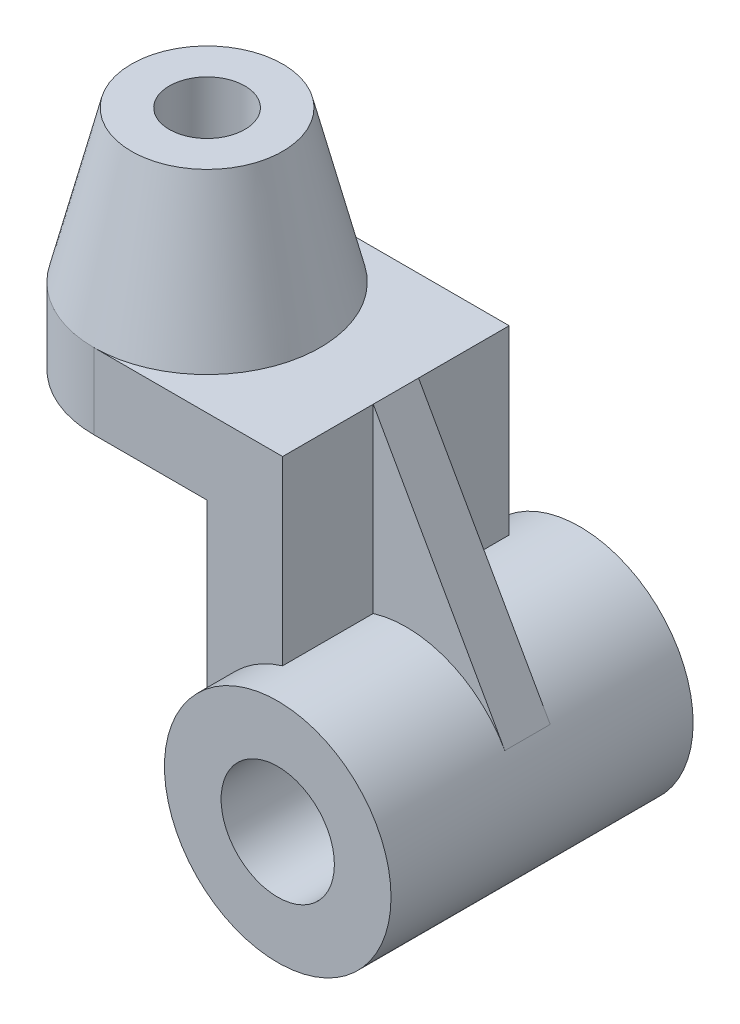
ISO-10303-21;
HEADER;
FILE_DESCRIPTION(('STEP AP214'),'2;1');
FILE_NAME('part.step','',(''),(''),'','','');
FILE_SCHEMA(('AUTOMOTIVE_DESIGN { 1 0 10303 214 1 1 1 1 }'));
ENDSEC;
DATA;
#1=APPLICATION_CONTEXT('core data for automotive mechanical design processes');
#2=APPLICATION_PROTOCOL_DEFINITION('international standard','automotive_design',2000,#1);
#3=PRODUCT_CONTEXT('',#1,'mechanical');
#4=PRODUCT('Part','Part','',(#3));
#5=PRODUCT_RELATED_PRODUCT_CATEGORY('part','',(#4));
#6=PRODUCT_DEFINITION_FORMATION('','',#4);
#7=PRODUCT_DEFINITION_CONTEXT('part definition',#1,'design');
#8=PRODUCT_DEFINITION('design','',#6,#7);
#9=PRODUCT_DEFINITION_SHAPE('','',#8);
#10=(LENGTH_UNIT() NAMED_UNIT(*) SI_UNIT(.MILLI.,.METRE.));
#11=(NAMED_UNIT(*) PLANE_ANGLE_UNIT() SI_UNIT($,.RADIAN.));
#12=(NAMED_UNIT(*) SI_UNIT($,.STERADIAN.) SOLID_ANGLE_UNIT());
#13=UNCERTAINTY_MEASURE_WITH_UNIT(LENGTH_MEASURE(1.E-05),#10,'distance_accuracy_value','');
#14=(GEOMETRIC_REPRESENTATION_CONTEXT(3) GLOBAL_UNCERTAINTY_ASSIGNED_CONTEXT((#13)) GLOBAL_UNIT_ASSIGNED_CONTEXT((#10,
#11,#12)) REPRESENTATION_CONTEXT('',''));
#15=CARTESIAN_POINT('',(0.,0.,0.));
#16=DIRECTION('',(0.,0.,1.));
#17=DIRECTION('',(1.,0.,0.));
#18=AXIS2_PLACEMENT_3D('',#15,#16,#17);
#19=CARTESIAN_POINT('',(-88.7082869338697,76.7082869338697,30.));
#20=DIRECTION('',(0.,-1.,0.));
#21=DIRECTION('',(1.,0.,0.));
#22=AXIS2_PLACEMENT_3D('',#19,#20,#21);
#23=PLANE('',#22);
#24=CARTESIAN_POINT('',(-58.7082869338697,76.7082869338697,0.));
#25=DIRECTION('',(0.,1.,0.));
#26=DIRECTION('',(-1.,0.,0.));
#27=AXIS2_PLACEMENT_3D('',#24,#25,#26);
#28=CIRCLE('',#27,30.);
#29=CARTESIAN_POINT('',(-58.7082869338697,76.7082869338697,30.));
#30=VERTEX_POINT('',#29);
#31=CARTESIAN_POINT('',(-58.7082869338697,76.7082869338697,-30.));
#32=VERTEX_POINT('',#31);
#33=EDGE_CURVE('E126',#30,#32,#28,.T.);
#34=ORIENTED_EDGE('',*,*,#33,.F.);
#35=DIRECTION('',(-1.,0.,0.));
#36=VECTOR('',#35,1.);
#37=CARTESIAN_POINT('',(-88.7082869338697,76.7082869338697,30.));
#38=LINE('',#37,#36);
#39=CARTESIAN_POINT('',(-8.7082869338697,76.7082869338697,30.));
#40=VERTEX_POINT('',#39);
#41=EDGE_CURVE('E109',#40,#30,#38,.T.);
#42=ORIENTED_EDGE('',*,*,#41,.F.);
#43=DIRECTION('',(0.,0.,-1.));
#44=VECTOR('',#43,1.);
#45=CARTESIAN_POINT('',(-8.7082869338697,76.7082869338697,30.));
#46=LINE('',#45,#44);
#47=CARTESIAN_POINT('',(-8.7082869338697,76.7082869338697,6.));
#48=VERTEX_POINT('',#47);
#49=EDGE_CURVE('E183',#40,#48,#46,.T.);
#50=ORIENTED_EDGE('',*,*,#49,.T.);
#51=DIRECTION('',(0.,0.,-1.));
#52=VECTOR('',#51,1.);
#53=CARTESIAN_POINT('',(-8.7082869338697,76.7082869338697,6.));
#54=LINE('',#53,#52);
#55=CARTESIAN_POINT('',(-8.7082869338697,76.7082869338697,-6.));
#56=VERTEX_POINT('',#55);
#57=EDGE_CURVE('E147',#48,#56,#54,.T.);
#58=ORIENTED_EDGE('',*,*,#57,.T.);
#59=CARTESIAN_POINT('',(-8.7082869338697,76.7082869338697,-30.));
#60=VERTEX_POINT('',#59);
#61=EDGE_CURVE('E184',#56,#60,#46,.T.);
#62=ORIENTED_EDGE('',*,*,#61,.T.);
#63=DIRECTION('',(-1.,0.,0.));
#64=VECTOR('',#63,1.);
#65=CARTESIAN_POINT('',(-88.7082869338697,76.7082869338697,-30.));
#66=LINE('',#65,#64);
#67=EDGE_CURVE('E128',#60,#32,#66,.T.);
#68=ORIENTED_EDGE('',*,*,#67,.T.);
#69=EDGE_LOOP('',(#34,#42,#50,#58,#62,#68));
#70=FACE_BOUND('',#69,.T.);
#71=ADVANCED_FACE('F39',(#70),#23,.F.);
#72=CARTESIAN_POINT('',(-28.7082869338697,56.7082869338697,30.));
#73=DIRECTION('',(0.,1.,0.));
#74=DIRECTION('',(-1.,0.,0.));
#75=AXIS2_PLACEMENT_3D('',#72,#73,#74);
#76=PLANE('',#75);
#77=CARTESIAN_POINT('',(-58.7082869338697,56.7082869338697,0.));
#78=DIRECTION('',(0.,1.,0.));
#79=DIRECTION('',(-1.,0.,0.));
#80=AXIS2_PLACEMENT_3D('',#77,#78,#79);
#81=CIRCLE('',#80,10.);
#82=CARTESIAN_POINT('',(-68.7082869338697,56.7082869338697,0.));
#83=VERTEX_POINT('',#82);
#84=EDGE_CURVE('E133',#83,#83,#81,.T.);
#85=ORIENTED_EDGE('',*,*,#84,.T.);
#86=EDGE_LOOP('',(#85));
#87=FACE_BOUND('',#86,.T.);
#88=CARTESIAN_POINT('',(-58.7082869338697,56.7082869338697,0.));
#89=DIRECTION('',(0.,1.,0.));
#90=DIRECTION('',(-1.,0.,0.));
#91=AXIS2_PLACEMENT_3D('',#88,#89,#90);
#92=CIRCLE('',#91,30.);
#93=CARTESIAN_POINT('',(-58.7082869338697,56.7082869338697,-30.));
#94=VERTEX_POINT('',#93);
#95=CARTESIAN_POINT('',(-58.7082869338697,56.7082869338697,30.));
#96=VERTEX_POINT('',#95);
#97=EDGE_CURVE('E53',#94,#96,#92,.T.);
#98=ORIENTED_EDGE('',*,*,#97,.F.);
#99=DIRECTION('',(1.,0.,0.));
#100=VECTOR('',#99,1.);
#101=CARTESIAN_POINT('',(-28.7082869338697,56.7082869338697,-30.));
#102=LINE('',#101,#100);
#103=CARTESIAN_POINT('',(-28.7082869338697,56.7082869338697,-30.));
#104=VERTEX_POINT('',#103);
#105=EDGE_CURVE('E177',#94,#104,#102,.T.);
#106=ORIENTED_EDGE('',*,*,#105,.T.);
#107=DIRECTION('',(0.,0.,-1.));
#108=VECTOR('',#107,1.);
#109=CARTESIAN_POINT('',(-28.7082869338697,56.7082869338697,30.));
#110=LINE('',#109,#108);
#111=CARTESIAN_POINT('',(-28.7082869338697,56.7082869338697,30.));
#112=VERTEX_POINT('',#111);
#113=EDGE_CURVE('E182',#112,#104,#110,.T.);
#114=ORIENTED_EDGE('',*,*,#113,.F.);
#115=DIRECTION('',(1.,0.,0.));
#116=VECTOR('',#115,1.);
#117=CARTESIAN_POINT('',(-28.7082869338697,56.7082869338697,30.));
#118=LINE('',#117,#116);
#119=EDGE_CURVE('E116',#96,#112,#118,.T.);
#120=ORIENTED_EDGE('',*,*,#119,.F.);
#121=EDGE_LOOP('',(#98,#106,#114,#120));
#122=FACE_BOUND('',#121,.T.);
#123=ADVANCED_FACE('F230',(#87,#122),#76,.F.);
#124=CARTESIAN_POINT('',(-8.7082869338697,76.7082869338697,30.));
#125=DIRECTION('',(-1.,0.,0.));
#126=DIRECTION('',(0.,-1.,0.));
#127=AXIS2_PLACEMENT_3D('',#124,#125,#126);
#128=PLANE('',#127);
#129=DIRECTION('',(0.,-1.,0.));
#130=VECTOR('',#129,1.);
#131=CARTESIAN_POINT('',(-8.7082869338697,76.7082869338697,-6.));
#132=LINE('',#131,#130);
#133=CARTESIAN_POINT('',(-8.7082869338697,28.7082869338697,-6.));
#134=VERTEX_POINT('',#133);
#135=EDGE_CURVE('E140',#56,#134,#132,.T.);
#136=ORIENTED_EDGE('',*,*,#135,.T.);
#137=DIRECTION('',(0.,0.,-1.));
#138=VECTOR('',#137,1.);
#139=CARTESIAN_POINT('',(-8.7082869338697,28.7082869338697,30.));
#140=LINE('',#139,#138);
#141=CARTESIAN_POINT('',(-8.7082869338697,28.7082869338697,-30.));
#142=VERTEX_POINT('',#141);
#143=EDGE_CURVE('E190',#134,#142,#140,.T.);
#144=ORIENTED_EDGE('',*,*,#143,.T.);
#145=DIRECTION('',(0.,1.,0.));
#146=VECTOR('',#145,1.);
#147=CARTESIAN_POINT('',(-8.7082869338697,76.7082869338697,-30.));
#148=LINE('',#147,#146);
#149=EDGE_CURVE('E175',#142,#60,#148,.T.);
#150=ORIENTED_EDGE('',*,*,#149,.T.);
#151=ORIENTED_EDGE('',*,*,#61,.F.);
#152=EDGE_LOOP('',(#136,#144,#150,#151));
#153=FACE_BOUND('',#152,.T.);
#154=ADVANCED_FACE('F225',(#153),#128,.F.);
#155=CARTESIAN_POINT('',(0.,0.,40.));
#156=DIRECTION('',(0.,0.,1.));
#157=DIRECTION('',(1.,0.,0.));
#158=AXIS2_PLACEMENT_3D('',#155,#156,#157);
#159=PLANE('',#158);
#160=CARTESIAN_POINT('',(0.,0.,40.));
#161=DIRECTION('',(0.,0.,1.));
#162=DIRECTION('',(1.,0.,0.));
#163=AXIS2_PLACEMENT_3D('',#160,#161,#162);
#164=CIRCLE('',#163,30.);
#165=CARTESIAN_POINT('',(30.,0.,40.));
#166=VERTEX_POINT('',#165);
#167=EDGE_CURVE('E121',#166,#166,#164,.T.);
#168=ORIENTED_EDGE('',*,*,#167,.T.);
#169=EDGE_LOOP('',(#168));
#170=FACE_BOUND('',#169,.T.);
#171=CARTESIAN_POINT('',(0.,0.,40.));
#172=DIRECTION('',(0.,0.,1.));
#173=DIRECTION('',(1.,0.,0.));
#174=AXIS2_PLACEMENT_3D('',#171,#172,#173);
#175=CIRCLE('',#174,15.);
#176=CARTESIAN_POINT('',(15.,0.,40.));
#177=VERTEX_POINT('',#176);
#178=EDGE_CURVE('E195',#177,#177,#175,.T.);
#179=ORIENTED_EDGE('',*,*,#178,.F.);
#180=EDGE_LOOP('',(#179));
#181=FACE_BOUND('',#180,.T.);
#182=ADVANCED_FACE('F210',(#170,#181),#159,.T.);
#183=CARTESIAN_POINT('',(0.,0.,-40.));
#184=DIRECTION('',(0.,0.,1.));
#185=DIRECTION('',(1.,0.,0.));
#186=AXIS2_PLACEMENT_3D('',#183,#184,#185);
#187=PLANE('',#186);
#188=CARTESIAN_POINT('',(0.,0.,-40.));
#189=DIRECTION('',(0.,0.,1.));
#190=DIRECTION('',(1.,0.,0.));
#191=AXIS2_PLACEMENT_3D('',#188,#189,#190);
#192=CIRCLE('',#191,30.);
#193=CARTESIAN_POINT('',(30.,0.,-40.));
#194=VERTEX_POINT('',#193);
#195=EDGE_CURVE('E191',#194,#194,#192,.T.);
#196=ORIENTED_EDGE('',*,*,#195,.F.);
#197=EDGE_LOOP('',(#196));
#198=FACE_BOUND('',#197,.T.);
#199=CARTESIAN_POINT('',(0.,0.,-40.));
#200=DIRECTION('',(0.,0.,1.));
#201=DIRECTION('',(1.,0.,0.));
#202=AXIS2_PLACEMENT_3D('',#199,#200,#201);
#203=CIRCLE('',#202,15.);
#204=CARTESIAN_POINT('',(15.,0.,-40.));
#205=VERTEX_POINT('',#204);
#206=EDGE_CURVE('E192',#205,#205,#203,.T.);
#207=ORIENTED_EDGE('',*,*,#206,.T.);
#208=EDGE_LOOP('',(#207));
#209=FACE_BOUND('',#208,.T.);
#210=ADVANCED_FACE('F204',(#198,#209),#187,.F.);
#211=CARTESIAN_POINT('',(0.,0.,40.));
#212=DIRECTION('',(0.,0.,-1.));
#213=DIRECTION('',(-1.,0.,0.));
#214=AXIS2_PLACEMENT_3D('',#211,#212,#213);
#215=CYLINDRICAL_SURFACE('',#214,30.);
#216=DIRECTION('',(0.,0.,-1.));
#217=VECTOR('',#216,1.);
#218=CARTESIAN_POINT('',(26.1508156568773,14.7015251072812,6.));
#219=LINE('',#218,#217);
#220=CARTESIAN_POINT('',(26.1508156568773,14.7015251072812,6.));
#221=VERTEX_POINT('',#220);
#222=CARTESIAN_POINT('',(26.1508156568773,14.7015251072812,-6.));
#223=VERTEX_POINT('',#222);
#224=EDGE_CURVE('E158',#221,#223,#219,.T.);
#225=ORIENTED_EDGE('',*,*,#224,.F.);
#226=CARTESIAN_POINT('',(0.,0.,6.));
#227=DIRECTION('',(0.,0.,1.));
#228=DIRECTION('',(1.,0.,0.));
#229=AXIS2_PLACEMENT_3D('',#226,#227,#228);
#230=CIRCLE('',#229,30.);
#231=CARTESIAN_POINT('',(-8.7082869338697,28.7082869338697,6.));
#232=VERTEX_POINT('',#231);
#233=EDGE_CURVE('E145',#221,#232,#230,.T.);
#234=ORIENTED_EDGE('',*,*,#233,.T.);
#235=CARTESIAN_POINT('',(-8.7082869338697,28.7082869338697,30.));
#236=VERTEX_POINT('',#235);
#237=EDGE_CURVE('E188',#236,#232,#140,.T.);
#238=ORIENTED_EDGE('',*,*,#237,.F.);
#239=CARTESIAN_POINT('',(0.,0.,30.));
#240=DIRECTION('',(0.,0.,-1.));
#241=DIRECTION('',(1.,0.,0.));
#242=AXIS2_PLACEMENT_3D('',#239,#240,#241);
#243=CIRCLE('',#242,30.);
#244=CARTESIAN_POINT('',(-28.7082869338697,8.7082869338697,30.));
#245=VERTEX_POINT('',#244);
#246=EDGE_CURVE('E161',#245,#236,#243,.T.);
#247=ORIENTED_EDGE('',*,*,#246,.F.);
#248=DIRECTION('',(0.,0.,-1.));
#249=VECTOR('',#248,1.);
#250=CARTESIAN_POINT('',(-28.7082869338697,8.70828693386971,30.));
#251=LINE('',#250,#249);
#252=CARTESIAN_POINT('',(-28.7082869338697,8.70828693386971,-30.));
#253=VERTEX_POINT('',#252);
#254=EDGE_CURVE('E166',#245,#253,#251,.T.);
#255=ORIENTED_EDGE('',*,*,#254,.T.);
#256=CARTESIAN_POINT('',(0.,0.,-30.));
#257=DIRECTION('',(0.,0.,-1.));
#258=DIRECTION('',(1.,0.,0.));
#259=AXIS2_PLACEMENT_3D('',#256,#257,#258);
#260=CIRCLE('',#259,30.);
#261=EDGE_CURVE('E159',#253,#142,#260,.T.);
#262=ORIENTED_EDGE('',*,*,#261,.T.);
#263=ORIENTED_EDGE('',*,*,#143,.F.);
#264=CARTESIAN_POINT('',(0.,0.,-6.));
#265=DIRECTION('',(0.,0.,1.));
#266=DIRECTION('',(1.,0.,0.));
#267=AXIS2_PLACEMENT_3D('',#264,#265,#266);
#268=CIRCLE('',#267,30.);
#269=EDGE_CURVE('E153',#223,#134,#268,.T.);
#270=ORIENTED_EDGE('',*,*,#269,.F.);
#271=EDGE_LOOP('',(#225,#234,#238,#247,#255,#262,#263,#270));
#272=FACE_BOUND('',#271,.T.);
#273=ORIENTED_EDGE('',*,*,#167,.F.);
#274=EDGE_LOOP('',(#273));
#275=FACE_BOUND('',#274,.T.);
#276=ORIENTED_EDGE('',*,*,#195,.T.);
#277=EDGE_LOOP('',(#276));
#278=FACE_BOUND('',#277,.T.);
#279=ADVANCED_FACE('F41',(#272,#275,#278),#215,.T.);
#280=CARTESIAN_POINT('',(0.,0.,40.));
#281=DIRECTION('',(0.,0.,-1.));
#282=DIRECTION('',(-1.,0.,0.));
#283=AXIS2_PLACEMENT_3D('',#280,#281,#282);
#284=CYLINDRICAL_SURFACE('',#283,15.);
#285=ORIENTED_EDGE('',*,*,#178,.T.);
#286=EDGE_LOOP('',(#285));
#287=FACE_BOUND('',#286,.T.);
#288=ORIENTED_EDGE('',*,*,#206,.F.);
#289=EDGE_LOOP('',(#288));
#290=FACE_BOUND('',#289,.T.);
#291=ADVANCED_FACE('F209',(#287,#290),#284,.F.);
#292=ORIENTED_EDGE('',*,*,#237,.T.);
#293=DIRECTION('',(0.,-1.,0.));
#294=VECTOR('',#293,1.);
#295=CARTESIAN_POINT('',(-8.7082869338697,76.7082869338697,6.));
#296=LINE('',#295,#294);
#297=EDGE_CURVE('E142',#48,#232,#296,.T.);
#298=ORIENTED_EDGE('',*,*,#297,.F.);
#299=ORIENTED_EDGE('',*,*,#49,.F.);
#300=DIRECTION('',(0.,1.,0.));
#301=VECTOR('',#300,1.);
#302=CARTESIAN_POINT('',(-8.7082869338697,76.7082869338697,30.));
#303=LINE('',#302,#301);
#304=EDGE_CURVE('E113',#236,#40,#303,.T.);
#305=ORIENTED_EDGE('',*,*,#304,.F.);
#306=EDGE_LOOP('',(#292,#298,#299,#305));
#307=FACE_BOUND('',#306,.T.);
#308=ADVANCED_FACE('F215',(#307),#128,.F.);
#309=CARTESIAN_POINT('',(-28.7082869338697,8.70828693386971,30.));
#310=DIRECTION('',(1.,0.,0.));
#311=DIRECTION('',(0.,0.,-1.));
#312=AXIS2_PLACEMENT_3D('',#309,#310,#311);
#313=PLANE('',#312);
#314=DIRECTION('',(0.,-1.,0.));
#315=VECTOR('',#314,1.);
#316=CARTESIAN_POINT('',(-28.7082869338697,8.70828693386971,-30.));
#317=LINE('',#316,#315);
#318=EDGE_CURVE('E162',#104,#253,#317,.T.);
#319=ORIENTED_EDGE('',*,*,#318,.T.);
#320=ORIENTED_EDGE('',*,*,#254,.F.);
#321=DIRECTION('',(0.,-1.,0.));
#322=VECTOR('',#321,1.);
#323=CARTESIAN_POINT('',(-28.7082869338697,8.70828693386971,30.));
#324=LINE('',#323,#322);
#325=EDGE_CURVE('E167',#112,#245,#324,.T.);
#326=ORIENTED_EDGE('',*,*,#325,.F.);
#327=ORIENTED_EDGE('',*,*,#113,.T.);
#328=EDGE_LOOP('',(#319,#320,#326,#327));
#329=FACE_BOUND('',#328,.T.);
#330=ADVANCED_FACE('F218',(#329),#313,.F.);
#331=CARTESIAN_POINT('',(0.,0.,30.));
#332=DIRECTION('',(0.,0.,1.));
#333=DIRECTION('',(1.,0.,0.));
#334=AXIS2_PLACEMENT_3D('',#331,#332,#333);
#335=PLANE('',#334);
#336=DIRECTION('',(0.,1.,0.));
#337=VECTOR('',#336,1.);
#338=CARTESIAN_POINT('',(-58.7082869338697,-30.,30.));
#339=LINE('',#338,#337);
#340=EDGE_CURVE('E50',#96,#30,#339,.T.);
#341=ORIENTED_EDGE('',*,*,#340,.F.);
#342=ORIENTED_EDGE('',*,*,#119,.T.);
#343=ORIENTED_EDGE('',*,*,#325,.T.);
#344=ORIENTED_EDGE('',*,*,#246,.T.);
#345=ORIENTED_EDGE('',*,*,#304,.T.);
#346=ORIENTED_EDGE('',*,*,#41,.T.);
#347=EDGE_LOOP('',(#341,#342,#343,#344,#345,#346));
#348=FACE_BOUND('',#347,.T.);
#349=ADVANCED_FACE('F112',(#348),#335,.T.);
#350=CARTESIAN_POINT('',(0.,0.,-30.));
#351=DIRECTION('',(0.,0.,1.));
#352=DIRECTION('',(1.,0.,0.));
#353=AXIS2_PLACEMENT_3D('',#350,#351,#352);
#354=PLANE('',#353);
#355=ORIENTED_EDGE('',*,*,#105,.F.);
#356=DIRECTION('',(0.,1.,0.));
#357=VECTOR('',#356,1.);
#358=CARTESIAN_POINT('',(-58.7082869338697,-30.,-30.));
#359=LINE('',#358,#357);
#360=EDGE_CURVE('E11',#94,#32,#359,.T.);
#361=ORIENTED_EDGE('',*,*,#360,.T.);
#362=ORIENTED_EDGE('',*,*,#67,.F.);
#363=ORIENTED_EDGE('',*,*,#149,.F.);
#364=ORIENTED_EDGE('',*,*,#261,.F.);
#365=ORIENTED_EDGE('',*,*,#318,.F.);
#366=EDGE_LOOP('',(#355,#361,#362,#363,#364,#365));
#367=FACE_BOUND('',#366,.T.);
#368=ADVANCED_FACE('F239',(#367),#354,.F.);
#369=CARTESIAN_POINT('',(-8.7082869338697,76.7082869338697,6.));
#370=DIRECTION('',(0.871693855229243,0.490050836909375,0.));
#371=DIRECTION('',(-0.490050836909375,0.871693855229244,0.));
#372=AXIS2_PLACEMENT_3D('',#369,#370,#371);
#373=PLANE('',#372);
#374=DIRECTION('',(0.490050836909375,-0.871693855229243,0.));
#375=VECTOR('',#374,1.);
#376=CARTESIAN_POINT('',(-8.7082869338697,76.7082869338697,-6.));
#377=LINE('',#376,#375);
#378=EDGE_CURVE('E65',#56,#223,#377,.T.);
#379=ORIENTED_EDGE('',*,*,#378,.F.);
#380=ORIENTED_EDGE('',*,*,#57,.F.);
#381=DIRECTION('',(0.490050836909375,-0.871693855229243,0.));
#382=VECTOR('',#381,1.);
#383=CARTESIAN_POINT('',(-8.7082869338697,76.7082869338697,6.));
#384=LINE('',#383,#382);
#385=EDGE_CURVE('E150',#48,#221,#384,.T.);
#386=ORIENTED_EDGE('',*,*,#385,.T.);
#387=ORIENTED_EDGE('',*,*,#224,.T.);
#388=EDGE_LOOP('',(#379,#380,#386,#387));
#389=FACE_BOUND('',#388,.T.);
#390=ADVANCED_FACE('F242',(#389),#373,.T.);
#391=CARTESIAN_POINT('',(0.,0.,6.));
#392=DIRECTION('',(0.,0.,1.));
#393=DIRECTION('',(1.,0.,0.));
#394=AXIS2_PLACEMENT_3D('',#391,#392,#393);
#395=PLANE('',#394);
#396=ORIENTED_EDGE('',*,*,#297,.T.);
#397=ORIENTED_EDGE('',*,*,#233,.F.);
#398=ORIENTED_EDGE('',*,*,#385,.F.);
#399=EDGE_LOOP('',(#396,#397,#398));
#400=FACE_BOUND('',#399,.T.);
#401=ADVANCED_FACE('F247',(#400),#395,.T.);
#402=CARTESIAN_POINT('',(0.,0.,-6.));
#403=DIRECTION('',(0.,0.,1.));
#404=DIRECTION('',(1.,0.,0.));
#405=AXIS2_PLACEMENT_3D('',#402,#403,#404);
#406=PLANE('',#405);
#407=ORIENTED_EDGE('',*,*,#135,.F.);
#408=ORIENTED_EDGE('',*,*,#378,.T.);
#409=ORIENTED_EDGE('',*,*,#269,.T.);
#410=EDGE_LOOP('',(#407,#408,#409));
#411=FACE_BOUND('',#410,.T.);
#412=ADVANCED_FACE('F250',(#411),#406,.F.);
#413=CARTESIAN_POINT('',(-58.7082869338697,-30.,0.));
#414=DIRECTION('',(0.,1.,0.));
#415=DIRECTION('',(-1.,0.,0.));
#416=AXIS2_PLACEMENT_3D('',#413,#414,#415);
#417=CYLINDRICAL_SURFACE('',#416,30.);
#418=ORIENTED_EDGE('',*,*,#97,.T.);
#419=ORIENTED_EDGE('',*,*,#340,.T.);
#420=CARTESIAN_POINT('',(-58.7082869338697,76.7082869338697,0.));
#421=DIRECTION('',(0.,1.,0.));
#422=DIRECTION('',(-1.,0.,0.));
#423=AXIS2_PLACEMENT_3D('',#420,#421,#422);
#424=CIRCLE('',#423,30.);
#425=EDGE_CURVE('E124',#32,#30,#424,.T.);
#426=ORIENTED_EDGE('',*,*,#425,.F.);
#427=ORIENTED_EDGE('',*,*,#360,.F.);
#428=EDGE_LOOP('',(#418,#419,#426,#427));
#429=FACE_BOUND('',#428,.T.);
#430=ADVANCED_FACE('F125',(#429),#417,.T.);
#431=CARTESIAN_POINT('',(-58.7082869338697,76.7082869338697,0.));
#432=DIRECTION('',(0.,-1.,0.));
#433=DIRECTION('',(-1.,0.,0.));
#434=AXIS2_PLACEMENT_3D('',#431,#432,#433);
#435=CONICAL_SURFACE('',#434,30.,0.244346095279207);
#436=CARTESIAN_POINT('',(-58.7082869338697,116.70828693387,0.));
#437=DIRECTION('',(0.,1.,0.));
#438=DIRECTION('',(-1.,0.,0.));
#439=AXIS2_PLACEMENT_3D('',#436,#437,#438);
#440=CIRCLE('',#439,20.0268798862728);
#441=CARTESIAN_POINT('',(-78.7351668201425,116.70828693387,0.));
#442=VERTEX_POINT('',#441);
#443=EDGE_CURVE('E135',#442,#442,#440,.T.);
#444=ORIENTED_EDGE('',*,*,#443,.F.);
#445=EDGE_LOOP('',(#444));
#446=FACE_BOUND('',#445,.T.);
#447=ORIENTED_EDGE('',*,*,#33,.T.);
#448=ORIENTED_EDGE('',*,*,#425,.T.);
#449=EDGE_LOOP('',(#447,#448));
#450=FACE_BOUND('',#449,.T.);
#451=ADVANCED_FACE('F131',(#446,#450),#435,.T.);
#452=CARTESIAN_POINT('',(-58.7082869338697,116.70828693387,0.));
#453=DIRECTION('',(0.,1.,0.));
#454=DIRECTION('',(-1.,0.,0.));
#455=AXIS2_PLACEMENT_3D('',#452,#453,#454);
#456=PLANE('',#455);
#457=CARTESIAN_POINT('',(-58.7082869338697,116.70828693387,0.));
#458=DIRECTION('',(0.,1.,0.));
#459=DIRECTION('',(-1.,0.,0.));
#460=AXIS2_PLACEMENT_3D('',#457,#458,#459);
#461=CIRCLE('',#460,10.);
#462=CARTESIAN_POINT('',(-68.7082869338697,116.70828693387,0.));
#463=VERTEX_POINT('',#462);
#464=EDGE_CURVE('E271',#463,#463,#461,.T.);
#465=ORIENTED_EDGE('',*,*,#464,.F.);
#466=EDGE_LOOP('',(#465));
#467=FACE_BOUND('',#466,.T.);
#468=ORIENTED_EDGE('',*,*,#443,.T.);
#469=EDGE_LOOP('',(#468));
#470=FACE_BOUND('',#469,.T.);
#471=ADVANCED_FACE('F256',(#467,#470),#456,.T.);
#472=CARTESIAN_POINT('',(-58.7082869338697,-30.,0.));
#473=DIRECTION('',(0.,1.,0.));
#474=DIRECTION('',(-1.,0.,0.));
#475=AXIS2_PLACEMENT_3D('',#472,#473,#474);
#476=CYLINDRICAL_SURFACE('',#475,10.);
#477=CARTESIAN_POINT('',(-68.7082869338697,116.70828693387,0.));
#478=CARTESIAN_POINT('',(-68.7082869338697,116.08328693387,0.));
#479=CARTESIAN_POINT('',(-68.7082869338697,115.45828693387,0.));
#480=CARTESIAN_POINT('',(-68.7082869338697,114.20828693387,0.));
#481=CARTESIAN_POINT('',(-68.7082869338697,113.58328693387,0.));
#482=CARTESIAN_POINT('',(-68.7082869338697,112.33328693387,0.));
#483=CARTESIAN_POINT('',(-68.7082869338697,111.70828693387,0.));
#484=CARTESIAN_POINT('',(-68.7082869338697,110.45828693387,0.));
#485=CARTESIAN_POINT('',(-68.7082869338697,109.83328693387,0.));
#486=CARTESIAN_POINT('',(-68.7082869338697,108.58328693387,0.));
#487=CARTESIAN_POINT('',(-68.7082869338697,107.95828693387,0.));
#488=CARTESIAN_POINT('',(-68.7082869338697,106.70828693387,0.));
#489=CARTESIAN_POINT('',(-68.7082869338697,106.08328693387,0.));
#490=CARTESIAN_POINT('',(-68.7082869338697,104.83328693387,0.));
#491=CARTESIAN_POINT('',(-68.7082869338697,104.20828693387,0.));
#492=CARTESIAN_POINT('',(-68.7082869338697,102.95828693387,0.));
#493=CARTESIAN_POINT('',(-68.7082869338697,102.33328693387,0.));
#494=CARTESIAN_POINT('',(-68.7082869338697,101.08328693387,0.));
#495=CARTESIAN_POINT('',(-68.7082869338697,100.45828693387,0.));
#496=CARTESIAN_POINT('',(-68.7082869338697,99.2082869338697,0.));
#497=CARTESIAN_POINT('',(-68.7082869338697,98.5832869338697,0.));
#498=CARTESIAN_POINT('',(-68.7082869338697,97.3332869338697,0.));
#499=CARTESIAN_POINT('',(-68.7082869338697,96.7082869338697,0.));
#500=CARTESIAN_POINT('',(-68.7082869338697,95.4582869338697,0.));
#501=CARTESIAN_POINT('',(-68.7082869338697,94.8332869338697,0.));
#502=CARTESIAN_POINT('',(-68.7082869338697,93.5832869338697,0.));
#503=CARTESIAN_POINT('',(-68.7082869338697,92.9582869338697,0.));
#504=CARTESIAN_POINT('',(-68.7082869338697,91.7082869338697,0.));
#505=CARTESIAN_POINT('',(-68.7082869338697,91.0832869338697,0.));
#506=CARTESIAN_POINT('',(-68.7082869338697,89.8332869338697,0.));
#507=CARTESIAN_POINT('',(-68.7082869338697,89.2082869338697,0.));
#508=CARTESIAN_POINT('',(-68.7082869338697,87.9582869338697,0.));
#509=CARTESIAN_POINT('',(-68.7082869338697,87.3332869338697,0.));
#510=CARTESIAN_POINT('',(-68.7082869338697,86.0832869338697,0.));
#511=CARTESIAN_POINT('',(-68.7082869338697,85.4582869338697,0.));
#512=CARTESIAN_POINT('',(-68.7082869338697,84.2082869338697,0.));
#513=CARTESIAN_POINT('',(-68.7082869338697,83.5832869338697,0.));
#514=CARTESIAN_POINT('',(-68.7082869338697,82.3332869338697,0.));
#515=CARTESIAN_POINT('',(-68.7082869338697,81.7082869338697,0.));
#516=CARTESIAN_POINT('',(-68.7082869338697,80.4582869338697,0.));
#517=CARTESIAN_POINT('',(-68.7082869338697,79.8332869338697,0.));
#518=CARTESIAN_POINT('',(-68.7082869338697,78.5832869338697,0.));
#519=CARTESIAN_POINT('',(-68.7082869338697,77.9582869338697,0.));
#520=CARTESIAN_POINT('',(-68.7082869338697,76.7082869338697,0.));
#521=CARTESIAN_POINT('',(-68.7082869338697,76.0832869338697,0.));
#522=CARTESIAN_POINT('',(-68.7082869338697,74.8332869338697,0.));
#523=CARTESIAN_POINT('',(-68.7082869338697,74.2082869338697,0.));
#524=CARTESIAN_POINT('',(-68.7082869338697,72.9582869338697,0.));
#525=CARTESIAN_POINT('',(-68.7082869338697,72.3332869338697,0.));
#526=CARTESIAN_POINT('',(-68.7082869338697,71.0832869338697,0.));
#527=CARTESIAN_POINT('',(-68.7082869338697,70.4582869338697,0.));
#528=CARTESIAN_POINT('',(-68.7082869338697,69.2082869338697,0.));
#529=CARTESIAN_POINT('',(-68.7082869338697,68.5832869338697,0.));
#530=CARTESIAN_POINT('',(-68.7082869338697,67.3332869338697,0.));
#531=CARTESIAN_POINT('',(-68.7082869338697,66.7082869338697,0.));
#532=CARTESIAN_POINT('',(-68.7082869338697,65.4582869338697,0.));
#533=CARTESIAN_POINT('',(-68.7082869338697,64.8332869338697,0.));
#534=CARTESIAN_POINT('',(-68.7082869338697,63.5832869338697,0.));
#535=CARTESIAN_POINT('',(-68.7082869338697,62.9582869338697,0.));
#536=CARTESIAN_POINT('',(-68.7082869338697,61.7082869338697,0.));
#537=CARTESIAN_POINT('',(-68.7082869338697,61.0832869338697,0.));
#538=CARTESIAN_POINT('',(-68.7082869338697,59.8332869338697,0.));
#539=CARTESIAN_POINT('',(-68.7082869338697,59.2082869338697,0.));
#540=CARTESIAN_POINT('',(-68.7082869338697,57.9582869338697,0.));
#541=CARTESIAN_POINT('',(-68.7082869338697,57.3332869338697,0.));
#542=CARTESIAN_POINT('',(-68.7082869338697,56.7082869338697,0.));
#543=B_SPLINE_CURVE_WITH_KNOTS('',3,(#477,#478,#479,#480,#481,#482,#483,#484,#485,#486,#487,
#488,#489,#490,#491,#492,#493,#494,#495,#496,#497,#498,#499,#500,#501,#502,#503,#504,#505,#506,
#507,#508,#509,#510,#511,#512,#513,#514,#515,#516,#517,#518,#519,#520,#521,#522,#523,#524,#525,
#526,#527,#528,#529,#530,#531,#532,#533,#534,#535,#536,#537,#538,#539,#540,#541,#542),
.UNSPECIFIED.,.F.,.F.,(4,2,2,2,2,2,2,2,2,2,2,2,2,2,2,2,2,2,2,2,2,2,2,2,2,2,2,2,2,2,2,2,4),(0.,
1.87499999999999,3.75,5.62499999999999,7.50000000000001,9.37499999999999,11.25,13.125,15.,
16.875,18.75,20.625,22.5,24.375,26.25,28.125,30.,31.875,33.75,35.625,37.5,39.375,41.25,43.125,
45.,46.875,48.75,50.625,52.5,54.375,56.25,58.125,60.),.UNSPECIFIED.);
#544=EDGE_CURVE('BSEAM265',#463,#83,#543,.T.);
#545=ORIENTED_EDGE('',*,*,#464,.T.);
#546=ORIENTED_EDGE('',*,*,#84,.F.);
#547=ORIENTED_EDGE('',*,*,#544,.T.);
#548=ORIENTED_EDGE('',*,*,#544,.F.);
#549=EDGE_LOOP('',(#545,#547,#546,#548));
#550=FACE_BOUND('',#549,.T.);
#551=ADVANCED_FACE('F265',(#550),#476,.F.);
#552=CLOSED_SHELL('',(#71,#123,#154,#182,#210,#279,#291,#308,#330,#349,#368,#390,#401,#412,#430,
#451,#471,#551));
#553=MANIFOLD_SOLID_BREP('B2',#552);
#554=ADVANCED_BREP_SHAPE_REPRESENTATION('',(#18,#553),#14);
#555=SHAPE_DEFINITION_REPRESENTATION(#9,#554);
ENDSEC;
END-ISO-10303-21;
